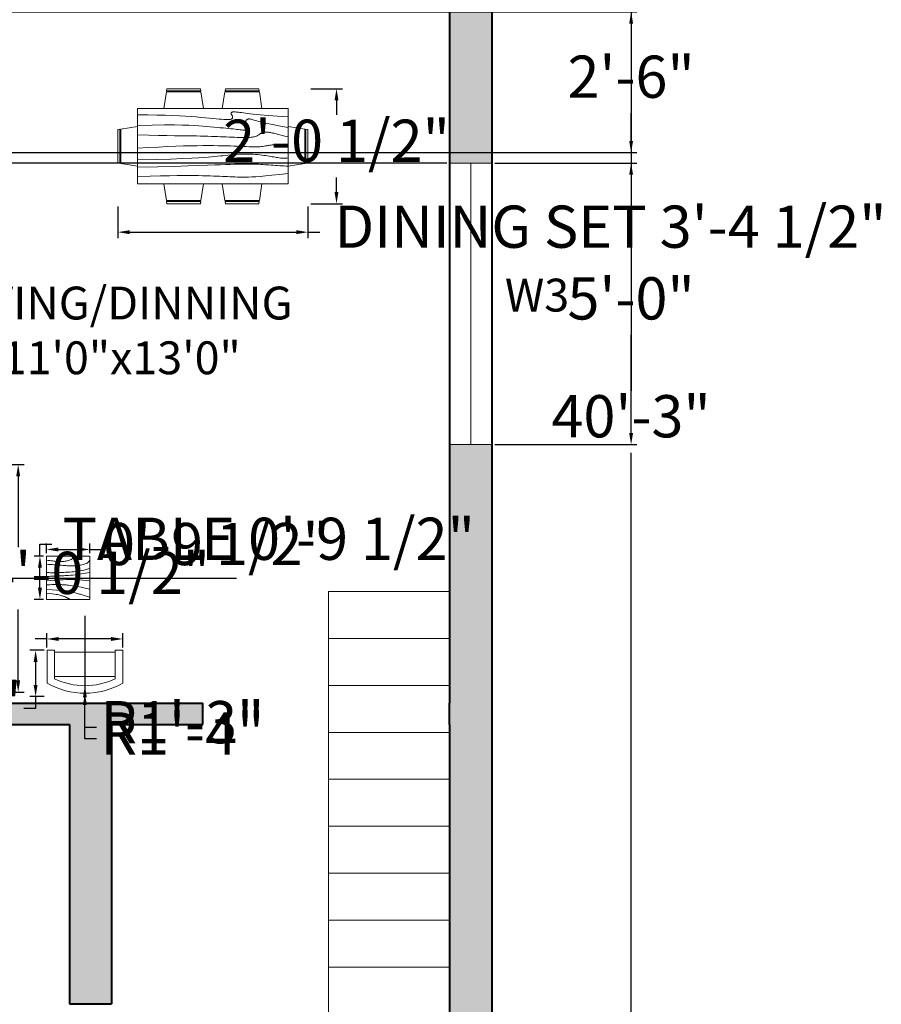
# Model space of a CAD drawing. Units: inches. Extents: x 1883 to 2353, y 1976 to 2541.
# Tile 4 of 5: x 2170 to 2353, y 2136 to 2346. Entities that reach past the tile are written whole.
import ezdxf

# ---------------------------------------------------------------- set-up
doc = ezdxf.new("R2010")
doc.units = ezdxf.units.IN
for name, color, linetype, lineweight in [('A-ANNO-DIMS', 2, 'Continuous', 18), ('A-ANNO-TEXT', 7, 'Continuous', 18), ('A-AREA-IDEN', 7, 'Continuous', 18), ('A-FLOR-STRS', 7, 'Continuous', 18), ('A-FURN', 8, 'Continuous', 18), ('A-GLAZ', 4, 'Continuous', 18), ('A-WALL', 7, 'Continuous', 40)]:
    doc.layers.add(name, color=color, linetype=linetype, lineweight=lineweight)
doc.layers.add('A-WALL-PATT', color=67, linetype='Continuous', lineweight=13, true_color=0x727430)
doc.styles.get("Standard").update_dxf_attribs({"font": 'arial.ttf'})
doc.dimstyles.new('ISO-25', dxfattribs={"dimtxt": 9, "dimasz": 2.5, "dimexe": 1.25, "dimexo": 0.625, "dimgap": 2, "dimtad": 0, "dimtih": 1, "dimtoh": 1, "dimdec": 1, "dimlunit": 4, "dimtxsty": 'Standard', "dimcen": 2.5, "dimadec": 0, "dimazin": 0, "dimtfac": 1, "dimtdec": 1, "dimtmove": 0, "dimatfit": 3, "dimfxl": 1, "dimarcsym": 0})

# ---------------------------------------------------------------- blocks, each defined once
blk = doc.blocks.new('Dining Set - 36 x 72 in.')
for p, q in [((-22.2343, 26.00059), (-23.4847, 17.99762)), ((-22.2304, 26), (-5.7608, 26)), ((-22, 27.5), (-22.1562, 26.50042)), ((-5.8416, 26.5), (-22.1534, 26.5)), ((-22, 27.5), (-6, 27.5)), ((-5.8437, 26.49966), (-6, 27.5)), ((-4.5152, 17.99762), (-5.7655, 25.99926)), ((5.7657, 26.00059), (4.5153, 17.99762)), ((5.7696, 26), (22.2392, 26)), ((6, 27.5), (5.8438, 26.50042)), ((22.1584, 26.5), (5.8466, 26.5)), ((6, 27.5), (22, 27.5)), ((22.1563, 26.49966), (22, 27.5)), ((23.4848, 17.99762), (22.2345, 25.99926)), ((36, 18), (-36, 18)), ((-36, 18), (-36, -18)), ((36, -18), (36, 18)), ((-44.0006, 8.23428), (-35.9976, 9.48474)), ((44.0006, 8.23428), (35.9976, 9.48474)), ((-45.5, 8), (-44.5004, 8.15617)), ((-45.5, 8), (-45.5, -8)), ((-44.5, -8.15843), (-44.5, 8.15338)), ((-44, 8.23041), (-44, -8.23915)), ((44, 8.23041), (44, -8.23915)), ((44.5, -8.15843), (44.5, 8.15338)), ((45.5, 8), (44.5005, 8.15617)), ((45.5, 8), (45.5, -8)), ((-44.4997, -8.15631), (-45.5, -8)), ((-35.9976, -9.48476), (-43.9993, -8.2345)), ((35.9976, -9.48476), (43.9993, -8.2345)), ((44.4997, -8.15631), (45.5, -8)), ((-36, -18), (36, -18)), ((-22.2343, -26.0006), (-23.4847, -17.99762)), ((-4.5152, -17.99762), (-5.7655, -25.99928)), ((5.7657, -26.0006), (4.5153, -17.99762)), ((23.4848, -17.99762), (22.2345, -25.99928)), ((-22.2304, -26), (-5.7608, -26)), ((-22, -27.5), (-22.1562, -26.50044)), ((-5.8416, -26.5), (-22.1534, -26.5)), ((-22, -27.5), (-6, -27.5)), ((-5.8437, -26.49967), (-6, -27.5)), ((5.7696, -26), (22.2392, -26)), ((6, -27.5), (5.8438, -26.50044)), ((22.1584, -26.5), (5.8466, -26.5)), ((6, -27.5), (22, -27.5)), ((22.1563, -26.49967), (22, -27.5))]:
    blk.add_line(p, q)
for points in [[(-36, 15), (-31.1772, 14.97754), (-26.8079, 14.91406), (-22.8538, 14.81543), (-19.276, 14.6875), (-16.0362, 14.53613), (-13.0957, 14.36718), (-10.4159, 14.18652), (-7.9583, 14), (-5.6904, 13.81315), (-3.6035, 13.63021), (-1.6954, 13.45508), (0.0365, 13.29166), (1.5945, 13.14388), (2.9811, 13.01562), (4.1988, 12.9108), (5.25, 12.83333), (6.1393, 12.78613), (6.8802, 12.76823), (7.4883, 12.77767), (7.9792, 12.8125), (8.3685, 12.87077), (8.6719, 12.95052), (8.9049, 13.0498), (9.0833, 13.16666), (9.2205, 13.29899), (9.3216, 13.44401), (9.3895, 13.59879), (9.4271, 13.76041), (9.4373, 13.92594), (9.4232, 14.09245), (9.3875, 14.257), (9.3333, 14.41666), (9.2638, 14.56917), (9.1836, 14.71484), (9.0975, 14.85465), (9.0104, 14.98958), (8.9272, 15.1206), (8.8529, 15.2487), (8.7922, 15.37483), (8.75, 15.5), (8.7305, 15.62467), (8.7344, 15.74739), (8.7617, 15.86621), (8.8125, 15.97916), (8.8867, 16.08431), (8.9844, 16.17968), (9.1055, 16.26334), (9.25, 16.33333), (9.4189, 16.38802), (9.6172, 16.42708), (9.8506, 16.45052), (10.125, 16.45833), (10.4463, 16.45052), (10.8203, 16.42708), (11.2529, 16.38802), (11.75, 16.33333), (12.3184, 16.26318), (12.9694, 16.17838), (13.7151, 16.07991), (14.5677, 15.96875), (15.5395, 15.84586), (16.6426, 15.71224), (17.8893, 15.56884), (19.2917, 15.41666), (20.859, 15.25667), (22.5879, 15.08984), (24.4721, 14.91715), (26.5052, 14.73958), (28.6809, 14.5581), (30.9929, 14.3737), (33.4347, 14.18733), (36, 14)], [(-36, 10), (-28.9766, 10.14274), (-23.1725, 10.20442), (-18.4241, 10.19775), (-14.5677, 10.13541), (-11.4399, 10.03011), (-8.877, 9.89453), (-6.7154, 9.74137), (-4.7917, 9.58333), (-2.9698, 9.43082), (-1.2246, 9.28515), (0.4415, 9.14534), (2.026, 9.01041), (3.5266, 8.87939), (4.9408, 8.7513), (6.266, 8.62516), (7.5, 8.5), (8.6411, 8.37549), (9.6914, 8.2539), (10.6538, 8.13818), (11.5312, 8.03125), (12.3267, 7.93603), (13.043, 7.85547), (13.6831, 7.79248), (14.25, 7.75), (14.7471, 7.7303), (15.1797, 7.73307), (15.5537, 7.75732), (15.875, 7.80208), (16.1494, 7.86637), (16.3828, 7.94922), (16.5811, 8.04964), (16.75, 8.16666), (16.8944, 8.29915), (17.0143, 8.44531), (17.1089, 8.60319), (17.1771, 8.77083), (17.218, 8.94629), (17.2305, 9.1276), (17.2137, 9.31282), (17.1667, 9.5), (17.0895, 9.6875), (16.987, 9.875), (16.8649, 10.0625), (16.7292, 10.25), (16.5856, 10.4375), (16.4401, 10.625), (16.2985, 10.8125), (16.1667, 11), (16.05, 11.18733), (15.9518, 11.3737), (15.8752, 11.5581), (15.8229, 11.73958), (15.798, 11.91715), (15.8034, 12.08984), (15.842, 12.25667), (15.9167, 12.41666), (16.0295, 12.56836), (16.1784, 12.70833), (16.3605, 12.83268), (16.5729, 12.9375), (16.8127, 13.01888), (17.0768, 13.07291), (17.3625, 13.0957), (17.6667, 13.08333), (17.9894, 13.03312), (18.3418, 12.94726), (18.7382, 12.82918), (19.1927, 12.68229), (19.7195, 12.51001), (20.3327, 12.31575), (21.0465, 12.10294), (21.875, 11.875), (22.8357, 11.63354), (23.959, 11.37304), (25.2786, 11.08618), (26.8282, 10.76562), (28.6414, 10.40405), (30.752, 9.99414), (33.1936, 9.52856), (36, 9)], [(-36, 5.5), (-30.7157, 5.3348), (-26.069, 5.20963), (-21.9946, 5.11767), (-18.4271, 5.05208), (-15.3009, 5.00602), (-12.5508, 4.97265), (-10.1112, 4.94515), (-7.9167, 4.91666), (-5.909, 4.88167), (-4.0586, 4.83984), (-2.3429, 4.79215), (-0.7396, 4.73958), (0.7739, 4.6831), (2.22, 4.6237), (3.6213, 4.56233), (5, 4.5), (6.373, 4.43782), (7.7344, 4.3776), (9.0723, 4.32129), (10.375, 4.27083), (11.6309, 4.22819), (12.8281, 4.19531), (13.9551, 4.17415), (15, 4.16666), (15.954, 4.17448), (16.819, 4.19791), (17.6001, 4.23698), (18.3021, 4.29166), (18.9299, 4.36198), (19.4883, 4.44791), (19.9823, 4.54948), (20.4167, 4.66666), (20.7969, 4.79899), (21.1302, 4.94401), (21.4245, 5.09879), (21.6875, 5.26041), (21.9271, 5.42594), (22.1511, 5.59245), (22.3672, 5.757), (22.5834, 5.91666), (22.8065, 6.06868), (23.0404, 6.21093), (23.2879, 6.34147), (23.5521, 6.45833), (23.8358, 6.55957), (24.142, 6.64323), (24.4735, 6.70735), (24.8334, 6.75), (25.2235, 6.76969), (25.642, 6.76692), (26.0858, 6.74267), (26.5521, 6.69791), (27.0379, 6.63362), (27.5404, 6.55078), (28.0565, 6.45036), (28.5834, 6.33333), (29.1242, 6.19987), (29.7071, 6.04687), (30.3661, 5.87044), (31.1354, 5.66666), (32.0493, 5.43164), (33.142, 5.16146), (34.4475, 4.85221), (36, 4.5)], [(-36, -1), (-30.7915, -0.6591), (-26.0195, -0.38216), (-21.6519, -0.16284), (-17.6563, 0.00521), (-14.0005, 0.12833), (-10.6523, 0.21289), (-7.5796, 0.26522), (-4.75, 0.29166), (-2.134, 0.29793), (0.2878, 0.28711), (2.5317, 0.26163), (4.6146, 0.22396), (6.5529, 0.17651), (8.3633, 0.12174), (10.0623, 0.06209), (11.6667, 0), (13.1899, -0.06201), (14.6341, -0.1211), (15.9982, -0.17432), (17.2813, -0.21875), (18.4823, -0.25147), (19.6003, -0.26953), (20.6343, -0.27002), (21.5834, -0.25), (22.4481, -0.20768), (23.2357, -0.14584), (23.9549, -0.06836), (24.6146, 0.02083), (25.2235, 0.11784), (25.7904, 0.21875), (26.3241, 0.31966), (26.8334, 0.41666), (27.3265, 0.50618), (27.8099, 0.58593), (28.2894, 0.65397), (28.7709, 0.70833), (29.2601, 0.74707), (29.763, 0.76823), (30.2855, 0.76985), (30.8334, 0.75), (31.4088, 0.70784), (31.9994, 0.64713), (32.589, 0.57275), (33.1615, 0.48958), (33.7008, 0.4025), (34.1908, 0.3164), (34.6153, 0.23616), (34.9584, 0.16666), (35.2099, 0.11165), (35.3848, 0.07031), (35.504, 0.04069), (35.5886, 0.02083), (35.6594, 0.00879), (35.7377, 0.0026), (35.8442, 0.00032), (36, 0)], [(-36, -6.5), (-27.1843, -6.31267), (-20.084, -6.1263), (-14.469, -5.9419), (-10.1094, -5.76042), (-6.7752, -5.58285), (-4.2363, -5.41016), (-2.2629, -5.24333), (-0.625, -5.08334), (0.8708, -4.93099), (2.2715, -4.78646), (3.5872, -4.64974), (4.8281, -4.52084), (6.0046, -4.39974), (7.127, -4.28646), (8.2053, -4.18099), (9.25, -4.08334), (10.2705, -3.99382), (11.2734, -3.91407), (12.2647, -3.84603), (13.25, -3.79167), (14.2354, -3.75293), (15.2266, -3.73177), (16.2295, -3.73015), (17.25, -3.75), (18.2912, -3.79248), (19.3451, -3.85547), (20.4009, -3.93604), (21.4479, -4.03125), (22.4754, -4.13819), (23.4727, -4.25391), (24.4289, -4.37549), (25.3334, -4.5), (26.1785, -4.62492), (26.9694, -4.74935), (27.7145, -4.87281), (28.4219, -4.99479), (29.1, -5.11483), (29.7572, -5.23242), (30.4016, -5.34709), (31.0417, -5.45834), (31.6837, -5.56437), (32.3262, -5.65821), (32.9658, -5.73153), (33.599, -5.77604), (34.2224, -5.78345), (34.8327, -5.74545), (35.4264, -5.65373), (36, -5.5)], [(-36, -10), (-26.4022, -9.81299), (-18.4675, -9.62891), (-11.9839, -9.45069), (-6.7396, -9.28125), (-2.5226, -9.12354), (0.8789, -8.98047), (3.6769, -8.85498), (6.0833, -8.75), (8.2767, -8.66765), (10.3021, -8.60677), (12.1712, -8.56543), (13.8958, -8.54167), (15.4876, -8.53353), (16.9583, -8.53907), (18.3197, -8.55632), (19.5834, -8.58334), (20.7616, -8.61841), (21.8685, -8.66081), (22.9188, -8.71004), (23.9271, -8.76563), (24.9081, -8.82707), (25.8763, -8.89388), (26.8465, -8.96558), (27.8334, -9.04167), (28.8474, -9.12118), (29.8828, -9.20117), (30.93, -9.27824), (31.9792, -9.34896), (33.0205, -9.40991), (34.0443, -9.45768), (35.0407, -9.48885), (36, -9.5)], [(-36, -14.5), (-30.0881, -14.33513), (-25.0332, -14.21224), (-20.7312, -14.12647), (-17.0781, -14.07292), (-13.97, -14.04671), (-11.3027, -14.04297), (-8.9724, -14.05681), (-6.875, -14.08334), (-4.9224, -14.11833), (-3.0905, -14.16016), (-1.3709, -14.20785), (0.2448, -14.26042), (1.7647, -14.3169), (3.1973, -14.3763), (4.5507, -14.43767), (5.8333, -14.5), (7.0554, -14.5621), (8.235, -14.62175), (9.3922, -14.67652), (10.5469, -14.72396), (11.7192, -14.76164), (12.929, -14.78711), (14.1965, -14.79794), (15.5417, -14.79167), (16.9933, -14.76424), (18.6152, -14.70508), (20.4804, -14.60197), (22.6615, -14.44271), (25.2312, -14.21509), (28.2624, -13.9069), (31.8277, -13.50594), (36, -13)]]:
    blk.add_lwpolyline(points)
blk = doc.blocks.new('Sofa - Roundback Loveseat 5 ft.')
for p, q in [((0, -32.44198), (0, -5.99998)), ((-24, -33.99998), (-24, -11.46958)), ((-23.9998, -13.38178), (23.99986, -13.38178)), ((24.00004, -33.99998), (24.00004, -11.46958)), ((-24, -32.44198), (24.00004, -32.44198))]:
    blk.add_line(p, q)
for points in [[(-24, -33.99998), (-30, -33.99998), (-30, -7.99998)], [(30.00004, -7.99998), (30.00004, -33.99998), (24.00004, -33.99998)]]:
    blk.add_lwpolyline(points)
for centre, radius, start, end in [((0, -60.24998), 60.24998, 60.13715, 119.8628), ((0, -61.38438), 55.38444, 64.32083, 115.6792)]:
    blk.add_arc(centre, radius, start, end)
blk = doc.blocks.new('Table - Square Woodgrain 42 x 42 in.')
blk.add_line((0, -42), (42, -42))
for points in [[(0, -4), (1.704, -4.2172), (3.2358, -4.4188), (4.615, -4.604), (5.8615, -4.7721), (6.9951, -4.9224), (8.0357, -5.0541), (9.0031, -5.1667), (9.9171, -5.2594), (10.7951, -5.3316), (11.6445, -5.3836), (12.4702, -5.4157), (13.277, -5.4283), (14.0698, -5.4217), (14.8535, -5.3964), (15.6331, -5.3526), (16.4133, -5.2908), (17.1986, -5.2103), (17.9913, -5.1062), (18.793, -4.9727), (19.6056, -4.8038), (20.4307, -4.5937), (21.2701, -4.3365), (22.1256, -4.0262), (22.9989, -3.6571), (23.888, -3.2272), (24.7756, -2.7516), (25.6408, -2.2491), (26.4624, -1.7387), (27.2195, -1.2395), (27.891, -0.7703), (28.456, -0.3501), (28.8934, 0.002)], [(0, -42), (0, 0), (42, 0), (42, -42)], [(0, -8), (1.8203, -8.1001), (3.6741, -8.2149), (5.5411, -8.3408), (7.4011, -8.4741), (9.2339, -8.6112), (11.0193, -8.7484), (12.7371, -8.8821), (14.3671, -9.0086), (15.8954, -9.1246), (17.3337, -9.2278), (18.6997, -9.3159), (20.0116, -9.387), (21.2871, -9.4389), (22.5442, -9.4696), (23.8008, -9.477), (25.0749, -9.459), (26.3791, -9.4137), (27.7049, -9.3403), (29.0383, -9.2382), (30.3655, -9.1068), (31.6728, -8.9455), (32.9461, -8.7535), (34.1717, -8.5304), (35.3358, -8.2756), (36.4268, -7.9863), (37.443, -7.6521), (38.3849, -7.2603), (39.253, -6.7986), (40.048, -6.2542), (40.7705, -5.6147), (41.421, -4.8674), (42, -4)], [(42, -12), (39.1784, -12.8621), (36.4519, -13.5654), (33.8246, -14.1294), (31.3004, -14.5731), (28.8832, -14.9161), (26.577, -15.1775), (24.3858, -15.3768), (22.3136, -15.5332), (20.3622, -15.6632), (18.5254, -15.7718), (16.7947, -15.8612), (15.1618, -15.9338), (13.6183, -15.9916), (12.1558, -16.0369), (10.7659, -16.0718), (9.4403, -16.0987), (8.1703, -16.1191), (6.9461, -16.1325), (5.7577, -16.1377), (4.595, -16.1335), (3.4479, -16.1188), (2.3064, -16.0924), (1.1604, -16.0532), (0, -16)], [(42, -16), (37.6529, -16.7365), (33.8802, -17.329), (30.6179, -17.7961), (27.8015, -18.1561), (25.3668, -18.4275), (23.2497, -18.6288), (21.3859, -18.7785), (19.7111, -18.8949), (18.1693, -18.9939), (16.7375, -19.0795), (15.401, -19.1534), (14.1449, -19.217), (12.9544, -19.2717), (11.8148, -19.3191), (10.7113, -19.3606), (9.6291, -19.3976), (8.5534, -19.4323), (7.47, -19.4689), (6.3643, -19.5122), (5.222, -19.5672), (4.0288, -19.6386), (2.7703, -19.7313), (1.4321, -19.8501), (0, -20)], [(0, -24), (3.9243, -23.6805), (7.4766, -23.4138), (10.6891, -23.1954), (13.5943, -23.0205), (16.2247, -22.8847), (18.6125, -22.7832), (20.7903, -22.7116), (22.7903, -22.6651), (24.6563, -22.642), (26.4764, -22.6507), (28.35, -22.7024), (30.3766, -22.8084), (32.6555, -22.98), (35.2861, -23.2283), (38.3678, -23.5645), (42, -24)], [(42, -32), (37.392, -31.017), (33.4585, -30.2231), (30.1291, -29.5949), (27.3334, -29.109), (25.0009, -28.742), (23.0612, -28.4707), (21.4439, -28.2716), (20.0786, -28.1215), (18.8998, -28.0002), (17.8609, -27.9014), (16.9206, -27.8219), (16.0371, -27.7588), (15.1691, -27.709), (14.2748, -27.6693), (13.3128, -27.6368), (12.2415, -27.6083), (11.0295, -27.5824), (9.6867, -27.5643), (8.233, -27.5608), (6.6884, -27.5787), (5.0728, -27.6248), (3.4062, -27.7058), (1.7086, -27.8286), (0, -28)], [(0, -32), (5.4026, -32.5358), (9.9494, -33.019), (13.7424, -33.4553), (16.8834, -33.8505), (19.4743, -34.2106), (21.6171, -34.5413), (23.4136, -34.8486), (24.9657, -35.1382), (26.3614, -35.4156), (27.6332, -35.6841), (28.7995, -35.9467), (29.8788, -36.2064), (30.8897, -36.4661), (31.8507, -36.7288), (32.7802, -36.9973), (33.6968, -37.2747), (34.6175, -37.5635), (35.5531, -37.8651), (36.5128, -38.1805), (37.506, -38.5108), (38.5421, -38.8568), (39.6302, -39.2197), (40.7797, -39.6004), (42, -40)], [(0, -36), (3.0098, -36.2857), (5.5354, -36.5643), (7.6368, -36.8359), (9.374, -37.1009), (10.807, -37.3597), (11.9957, -37.6126), (13.0002, -37.8599), (13.8804, -38.102), (14.6874, -38.3393), (15.4365, -38.5729), (16.1338, -38.8041), (16.7858, -39.0341), (17.3987, -39.264), (17.9787, -39.4952), (18.5322, -39.7288), (19.0655, -39.9662), (19.5832, -40.2081), (20.0842, -40.4544), (20.5657, -40.7046), (21.0249, -40.9581), (21.459, -41.2144), (21.8653, -41.4731), (22.2409, -41.7335), (22.5831, -41.9951)]]:
    blk.add_lwpolyline(points)
blk = doc.blocks.new('*D31')
at = {"layer": 'A-ANNO-DIMS', "color": 0, "lineweight": -2, "transparency": 16777216}
for p, q in [((2190.81, 2306.42), (2190.81, 2299.72)), ((2231.31, 2306.42), (2231.31, 2299.72)), ((2193.31, 2300.97), (2228.81, 2300.97)), ((2231.31, 2300.97), (2233.81, 2300.97))]:
    blk.add_line(p, q, dxfattribs=at)
at = {"layer": 'A-ANNO-DIMS', "color": 0, "transparency": 16777216}
for points in [[(2193.31, 2301.38), (2193.31, 2300.55), (2190.81, 2300.97)], [(2228.81, 2301.38), (2228.81, 2300.55), (2231.31, 2300.97)]]:
    blk.add_solid(points, dxfattribs=at)
at = {"layer": 'Defpoints', "color": 0, "transparency": 16777216}
for p in [(2190.81, 2307.04), (2231.31, 2307.04), (2231.31, 2300.97)]:
    blk.add_point(p, dxfattribs=at)
at = {"layer": 'A-ANNO-DIMS', "color": 0, "transparency": 16777216, "insert": (2295.76, 2300.97), "char_height": 9, "attachment_point": 5}
blk.add_mtext('DINING SET 3\'-4 1/2"', dxfattribs=at)
blk = doc.blocks.new('*D32')
at = {"layer": 'A-ANNO-DIMS', "color": 0, "lineweight": -2, "transparency": 16777216}
for p, q in [((2231.94, 2331.53), (2238.64, 2331.53)), ((2237.39, 2329.03), (2237.39, 2325.94)), ((2237.39, 2309.54), (2237.39, 2312.63)), ((2231.94, 2307.04), (2238.64, 2307.04))]:
    blk.add_line(p, q, dxfattribs=at)
at = {"layer": 'A-ANNO-DIMS', "color": 0, "transparency": 16777216}
for points in [[(2236.97, 2329.03), (2237.81, 2329.03), (2237.39, 2331.53)], [(2236.97, 2309.54), (2237.81, 2309.54), (2237.39, 2307.04)]]:
    blk.add_solid(points, dxfattribs=at)
at = {"layer": 'Defpoints', "color": 0, "transparency": 16777216}
for p in [(2231.31, 2331.53), (2237.39, 2331.53), (2231.31, 2307.04)]:
    blk.add_point(p, dxfattribs=at)
at = {"layer": 'A-ANNO-DIMS', "color": 0, "transparency": 16777216, "insert": (2237.39, 2319.28), "char_height": 9, "attachment_point": 5}
blk.add_mtext('2\'-0 1/2"', dxfattribs=at)
blk = doc.blocks.new('*D33')
at = {"layer": 'A-ANNO-DIMS', "color": 0, "lineweight": -2, "transparency": 16777216}
for p, q in [((2162.94, 2251.43), (2170.84, 2251.43)), ((2169.59, 2248.93), (2169.59, 2233.85)), ((2169.59, 2205.45), (2169.59, 2220.53)), ((2162.94, 2202.95), (2170.84, 2202.95))]:
    blk.add_line(p, q, dxfattribs=at)
at = {"layer": 'A-ANNO-DIMS', "color": 0, "transparency": 16777216}
for points in [[(2169.17, 2248.93), (2170.01, 2248.93), (2169.59, 2251.43)], [(2169.17, 2205.45), (2170.01, 2205.45), (2169.59, 2202.95)]]:
    blk.add_solid(points, dxfattribs=at)
at = {"layer": 'Defpoints', "color": 0, "transparency": 16777216}
for p in [(2162.32, 2251.43), (2169.59, 2251.43), (2162.32, 2202.95)]:
    blk.add_point(p, dxfattribs=at)
at = {"layer": 'A-ANNO-DIMS', "color": 0, "transparency": 16777216, "insert": (2169.59, 2227.19), "char_height": 9, "attachment_point": 5}
blk.add_mtext('SOFA 4\'-0 1/2"', dxfattribs=at)
blk = doc.blocks.new('*D35')
at = {"layer": 'A-ANNO-DIMS', "color": 0, "lineweight": -2, "transparency": 16777216}
for p, q in [((2175.72, 2214.27), (2173.22, 2214.27)), ((2175.72, 2212.47), (2175.72, 2215.52)), ((2189.37, 2214.27), (2178.22, 2214.27)), ((2191.87, 2212.47), (2191.87, 2215.52))]:
    blk.add_line(p, q, dxfattribs=at)
at = {"layer": 'A-ANNO-DIMS', "color": 0, "transparency": 16777216}
for points in [[(2178.22, 2214.69), (2178.22, 2213.85), (2175.72, 2214.27)], [(2189.37, 2214.69), (2189.37, 2213.85), (2191.87, 2214.27)]]:
    blk.add_solid(points, dxfattribs=at)
at = {"layer": 'Defpoints', "color": 0, "transparency": 16777216}
for p in [(2175.72, 2214.27), (2175.72, 2211.85), (2191.87, 2211.85)]:
    blk.add_point(p, dxfattribs=at)
at = {"layer": 'A-ANNO-DIMS', "color": 0, "transparency": 16777216, "insert": (2124.52, 2214.27), "char_height": 9, "attachment_point": 5}
blk.add_mtext('LOVESEAT 1\'-4"', dxfattribs=at)
blk = doc.blocks.new('*D36')
at = {"layer": 'A-ANNO-DIMS', "color": 0, "lineweight": -2, "transparency": 16777216}
for p, q in [((2175.1, 2211.85), (2172.05, 2211.85)), ((2173.3, 2209.35), (2173.3, 2204.48)), ((2175.1, 2201.98), (2172.05, 2201.98)), ((2173.3, 2201.98), (2173.3, 2199.48)), ((2173.3, 2199.48), (2170.8, 2199.48))]:
    blk.add_line(p, q, dxfattribs=at)
at = {"layer": 'A-ANNO-DIMS', "color": 0, "transparency": 16777216}
for points in [[(2172.88, 2209.35), (2173.72, 2209.35), (2173.3, 2211.85)], [(2172.88, 2204.48), (2173.72, 2204.48), (2173.3, 2201.98)]]:
    blk.add_solid(points, dxfattribs=at)
at = {"layer": 'Defpoints', "color": 0, "transparency": 16777216}
for p in [(2175.72, 2211.85), (2173.3, 2201.98), (2175.72, 2201.98)]:
    blk.add_point(p, dxfattribs=at)
at = {"layer": 'A-ANNO-DIMS', "color": 0, "transparency": 16777216, "insert": (2153.34, 2199.48), "char_height": 9, "attachment_point": 5}
blk.add_mtext('0\'-10"', dxfattribs=at)
blk = doc.blocks.new('*D37')
at = {"layer": 'A-ANNO-DIMS', "color": 0, "lineweight": -2, "transparency": 16777216}
for p, q in [((2174.22, 2231.95), (2174.22, 2234.45)), ((2174.22, 2234.45), (2176.72, 2234.45)), ((2174.99, 2231.95), (2172.97, 2231.95)), ((2174.22, 2225.19), (2174.22, 2229.45)), ((2174.99, 2222.69), (2172.97, 2222.69))]:
    blk.add_line(p, q, dxfattribs=at)
at = {"layer": 'A-ANNO-DIMS', "color": 0, "transparency": 16777216}
for points in [[(2173.8, 2229.45), (2174.64, 2229.45), (2174.22, 2231.95)], [(2173.8, 2225.19), (2174.64, 2225.19), (2174.22, 2222.69)]]:
    blk.add_solid(points, dxfattribs=at)
at = {"layer": 'Defpoints', "color": 0, "transparency": 16777216}
for p in [(2174.22, 2231.95), (2175.61, 2231.95), (2175.61, 2222.69)]:
    blk.add_point(p, dxfattribs=at)
at = {"layer": 'A-ANNO-DIMS', "color": 0, "transparency": 16777216, "insert": (2222.94, 2234.45), "char_height": 9, "attachment_point": 5}
blk.add_mtext('TABLE 0\'-9 1/2"', dxfattribs=at)
blk = doc.blocks.new('*D38')
at = {"layer": 'A-ANNO-DIMS', "color": 0, "lineweight": -2, "transparency": 16777216}
for p, q in [((2175.61, 2232.58), (2175.61, 2234.59)), ((2178.11, 2233.34), (2182.37, 2233.34)), ((2184.87, 2232.58), (2184.87, 2234.59)), ((2184.87, 2233.34), (2187.37, 2233.34))]:
    blk.add_line(p, q, dxfattribs=at)
at = {"layer": 'A-ANNO-DIMS', "color": 0, "transparency": 16777216}
for points in [[(2178.11, 2233.76), (2178.11, 2232.93), (2175.61, 2233.34)], [(2182.37, 2233.76), (2182.37, 2232.93), (2184.87, 2233.34)]]:
    blk.add_solid(points, dxfattribs=at)
at = {"layer": 'Defpoints', "color": 0, "transparency": 16777216}
for p in [(2184.87, 2233.34), (2175.61, 2231.95), (2184.87, 2231.95)]:
    blk.add_point(p, dxfattribs=at)
at = {"layer": 'A-ANNO-DIMS', "color": 0, "transparency": 16777216, "insert": (2211.82, 2233.34), "char_height": 9, "attachment_point": 5}
blk.add_mtext('0\'-9 1/2"', dxfattribs=at)
blk = doc.blocks.new('*D43')
at = {"layer": 'A-ANNO-DIMS', "color": 0, "lineweight": -2, "transparency": 16777216}
for p, q in [((2271.12, 2502.07), (2301.39, 2502.07)), ((2300.14, 2499.57), (2300.14, 2267.17)), ((2300.14, 2021.57), (2300.14, 2253.97)), ((2271.12, 2019.07), (2301.39, 2019.07))]:
    blk.add_line(p, q, dxfattribs=at)
at = {"layer": 'A-ANNO-DIMS', "color": 0, "transparency": 16777216}
for points in [[(2299.73, 2499.57), (2300.56, 2499.57), (2300.14, 2502.07)], [(2299.73, 2021.57), (2300.56, 2021.57), (2300.14, 2019.07)]]:
    blk.add_solid(points, dxfattribs=at)
at = {"layer": 'Defpoints', "color": 0, "transparency": 16777216}
for p in [(2270.49, 2502.07), (2300.14, 2502.07), (2270.49, 2019.07)]:
    blk.add_point(p, dxfattribs=at)
at = {"layer": 'A-ANNO-DIMS', "color": 0, "transparency": 16777216, "insert": (2300.14, 2260.57), "char_height": 9, "attachment_point": 5}
blk.add_mtext('40\'-3"', dxfattribs=at)
blk = doc.blocks.new('*D47')
at = {"layer": 'A-ANNO-DIMS', "color": 0, "lineweight": -2, "transparency": 16777216}
for p, q in [((2271.12, 2315.69), (2301.39, 2315.69)), ((2300.14, 2313.19), (2300.14, 2292.28)), ((2300.14, 2258.19), (2300.14, 2279.09)), ((2271.12, 2255.69), (2301.39, 2255.69))]:
    blk.add_line(p, q, dxfattribs=at)
at = {"layer": 'A-ANNO-DIMS', "color": 0, "transparency": 16777216}
for points in [[(2299.73, 2313.19), (2300.56, 2313.19), (2300.14, 2315.69)], [(2299.73, 2258.19), (2300.56, 2258.19), (2300.14, 2255.69)]]:
    blk.add_solid(points, dxfattribs=at)
at = {"layer": 'Defpoints', "color": 0, "transparency": 16777216}
for p in [(2270.49, 2315.69), (2300.14, 2315.69), (2270.49, 2255.69)]:
    blk.add_point(p, dxfattribs=at)
at = {"layer": 'A-ANNO-DIMS', "color": 0, "transparency": 16777216, "insert": (2300.14, 2285.69), "char_height": 9, "attachment_point": 5}
blk.add_mtext('5\'-0"', dxfattribs=at)
blk = doc.blocks.new('*D48')
at = {"layer": 'A-ANNO-DIMS', "color": 0, "lineweight": -2, "transparency": 16777216}
for p, q in [((2260.87, 2356.57), (1979.44, 2356.57)), ((1980.69, 2354.07), (1980.69, 2342.73)), ((1980.69, 2318.19), (1980.69, 2329.53)), ((2260.87, 2315.69), (1979.44, 2315.69))]:
    blk.add_line(p, q, dxfattribs=at)
at = {"layer": 'A-ANNO-DIMS', "color": 0, "transparency": 16777216}
for points in [[(1980.28, 2354.07), (1981.11, 2354.07), (1980.69, 2356.57)], [(1980.28, 2318.19), (1981.11, 2318.19), (1980.69, 2315.69)]]:
    blk.add_solid(points, dxfattribs=at)
at = {"layer": 'Defpoints', "color": 0, "transparency": 16777216}
for p in [(1980.69, 2356.57), (2261.49, 2356.57), (2261.49, 2315.69)]:
    blk.add_point(p, dxfattribs=at)
at = {"layer": 'A-ANNO-DIMS', "color": 0, "transparency": 16777216, "insert": (1980.69, 2336.13), "char_height": 9, "attachment_point": 5}
blk.add_mtext('3\'-5"', dxfattribs=at)
blk = doc.blocks.new('*D54')
at = {"layer": 'A-ANNO-DIMS', "color": 0, "lineweight": -2, "transparency": 16777216}
for p, q in [((2100.12, 2347.93), (2301.39, 2347.93)), ((2300.14, 2345.43), (2300.14, 2339.52)), ((2300.14, 2320.43), (2300.14, 2326.33)), ((2100.12, 2317.93), (2301.39, 2317.93))]:
    blk.add_line(p, q, dxfattribs=at)
at = {"layer": 'A-ANNO-DIMS', "color": 0, "transparency": 16777216}
for points in [[(2299.73, 2345.43), (2300.56, 2345.43), (2300.14, 2347.93)], [(2299.73, 2320.43), (2300.56, 2320.43), (2300.14, 2317.93)]]:
    blk.add_solid(points, dxfattribs=at)
at = {"layer": 'Defpoints', "color": 0, "transparency": 16777216}
for p in [(2099.49, 2347.93), (2300.14, 2347.93), (2099.49, 2317.93)]:
    blk.add_point(p, dxfattribs=at)
at = {"layer": 'A-ANNO-DIMS', "color": 0, "transparency": 16777216, "insert": (2300.14, 2332.93), "char_height": 9, "attachment_point": 5}
blk.add_mtext('2\'-6"', dxfattribs=at)
blk = doc.blocks.new('*D64')
at = {"layer": 'A-ANNO-DIMS', "color": 0, "lineweight": -2, "transparency": 16777216}
for p, q in [((2104.18, 2227.19), (2143.66, 2227.19)), ((2216.11, 2227.19), (2146.16, 2227.19))]:
    blk.add_line(p, q, dxfattribs=at)
at = {"layer": 'A-ANNO-DIMS', "color": 0, "transparency": 16777216}
blk.add_solid([(2143.66, 2227.61), (2143.66, 2226.77), (2146.16, 2227.19)], dxfattribs=at)
at = {"layer": 'Defpoints', "color": 0, "transparency": 16777216}
for p in [(2146.16, 2227.19), (2216.11, 2227.19)]:
    blk.add_point(p, dxfattribs=at)
at = {"layer": 'A-ANNO-DIMS', "color": 0, "transparency": 16777216, "insert": (2082.42, 2227.19), "char_height": 9, "attachment_point": 5}
blk.add_mtext('R5\'-10"', dxfattribs=at)
blk = doc.blocks.new('*D65')
at = {"layer": 'A-ANNO-DIMS', "color": 0, "lineweight": -2, "transparency": 16777216}
for p, q in [((2103.13, 2227.19), (2140.19, 2227.19)), ((2208.64, 2227.19), (2142.69, 2227.19))]:
    blk.add_line(p, q, dxfattribs=at)
at = {"layer": 'A-ANNO-DIMS', "color": 0, "transparency": 16777216}
blk.add_solid([(2140.19, 2227.61), (2140.19, 2226.77), (2142.69, 2227.19)], dxfattribs=at)
at = {"layer": 'Defpoints', "color": 0, "transparency": 16777216}
for p in [(2142.69, 2227.19), (2208.64, 2227.19)]:
    blk.add_point(p, dxfattribs=at)
at = {"layer": 'A-ANNO-DIMS', "color": 0, "transparency": 16777216, "insert": (2084.86, 2227.19), "char_height": 9, "attachment_point": 5}
blk.add_mtext('R5\'-6"', dxfattribs=at)
blk = doc.blocks.new('*D66')
at = {"layer": 'A-ANNO-DIMS', "color": 0, "lineweight": -2, "transparency": 16777216}
for p, q in [((2183.8, 2218.91), (2183.8, 2202.7)), ((2183.8, 2192.97), (2183.8, 2200.2)), ((2186.3, 2192.97), (2183.8, 2192.97))]:
    blk.add_line(p, q, dxfattribs=at)
at = {"layer": 'A-ANNO-DIMS', "color": 0, "transparency": 16777216}
blk.add_solid([(2184.21, 2200.2), (2183.38, 2200.2), (2183.8, 2202.7)], dxfattribs=at)
at = {"layer": 'Defpoints', "color": 0, "transparency": 16777216}
for p in [(2183.8, 2218.91), (2183.8, 2202.7)]:
    blk.add_point(p, dxfattribs=at)
at = {"layer": 'A-ANNO-DIMS', "color": 0, "transparency": 16777216, "insert": (2204.57, 2192.97), "char_height": 9, "attachment_point": 5}
blk.add_mtext('R1\'-4"', dxfattribs=at)
blk = doc.blocks.new('*D67')
at = {"layer": 'A-ANNO-DIMS', "color": 0, "lineweight": -2, "transparency": 16777216}
for p, q in [((2183.8, 2219.22), (2183.8, 2204.31)), ((2183.8, 2195.37), (2183.8, 2201.81)), ((2186.3, 2195.37), (2183.8, 2195.37))]:
    blk.add_line(p, q, dxfattribs=at)
at = {"layer": 'A-ANNO-DIMS', "color": 0, "transparency": 16777216}
blk.add_solid([(2184.21, 2201.81), (2183.38, 2201.81), (2183.8, 2204.31)], dxfattribs=at)
at = {"layer": 'Defpoints', "color": 0, "transparency": 16777216}
for p in [(2183.8, 2219.22), (2183.8, 2204.31)]:
    blk.add_point(p, dxfattribs=at)
at = {"layer": 'A-ANNO-DIMS', "color": 0, "transparency": 16777216, "insert": (2204.57, 2195.37), "char_height": 9, "attachment_point": 5}
blk.add_mtext('R1\'-3"', dxfattribs=at)

msp = doc.modelspace()

# ---------------------------------------------------------------- hatches: boundary and pattern name
at = {"layer": 'A-WALL-PATT'}
h = msp.add_hatch(color=256, dxfattribs=at)
h.dxf.hatch_style = 1
h.paths.add_polyline_path([(2057.49, 2502.07), (2006.49, 2502.07), (2006.49, 2344.57), (2015.49, 2344.57), (2015.49, 2356.57), (2099.49, 2356.57), (2099.49, 2347.93), (2103.99, 2347.93), (2103.99, 2356.57), (2108.06, 2356.57, -0.029386), (2108.06, 2361.07), (2015.49, 2361.07), (2015.49, 2493.07), (2057.49, 2493.07)])
h.paths.add_polyline_path([(2182.74, 2502.07), (2105.49, 2502.07), (2105.49, 2493.07), (2147.49, 2493.07), (2147.49, 2361.07), (2144.06, 2361.07), (2144.06, 2356.57), (2151.99, 2356.57), (2155, 2356.57), (2155, 2361.07), (2151.99, 2361.07), (2151.99, 2493.07), (2182.74, 2493.07)])
h.paths.add_polyline_path([(2270.49, 2502.07), (2230.74, 2502.07), (2230.74, 2493.07), (2261.49, 2493.07), (2261.49, 2361.07), (2191, 2361.07, -0.029386), (2191, 2356.57), (2261.49, 2356.57), (2261.49, 2315.69), (2270.49, 2315.69)])
h.paths.add_polyline_path([(2051.49, 2131.57), (2015.49, 2131.57), (2015.49, 2251.57), (2103.99, 2251.57), (2104.81, 2251.57, -0.028441), (2104.81, 2256.07), (2103.99, 2256.07), (2103.99, 2260.88), (2099.49, 2260.88), (2099.49, 2256.07), (2015.49, 2256.07), (2015.49, 2268.07), (2006.49, 2268.07), (2006.49, 2122.57), (2015.49, 2122.57), (2051.49, 2122.57)])
h.paths.add_polyline_path([(2103.99, 2308.57), (2103.99, 2317.93, -0.034841), (2099.49, 2317.93), (2099.49, 2308.57), (2015.49, 2308.57), (2015.49, 2320.57), (2006.49, 2320.57), (2006.49, 2292.07), (2015.49, 2292.07), (2015.49, 2304.07), (2099.49, 2304.07), (2099.49, 2290.88, -0.034841), (2103.99, 2290.88), (2103.99, 2304.07)])
h = msp.add_hatch(color=256, dxfattribs=at)
h.dxf.hatch_style = 1
h.paths.add_polyline_path([(2189.49, 2090.74), (2180.49, 2090.74), (2180.49, 2071.57, -0.034524), (2180.49, 2067.07), (2189.49, 2067.07), (2261.49, 2067.07), (2270.49, 2067.07), (2270.49, 2094.07), (2270.49, 2255.69), (2261.49, 2255.69), (2261.49, 2200.57), (2261.49, 2196.07), (2261.49, 2094.07), (2261.49, 2076.07), (2189.49, 2076.07)])
h.paths.add_polyline_path([(2189.49, 2196.07), (2208.94, 2196.07), (2208.94, 2200.57), (2151.99, 2200.57), (2139.99, 2200.57), (2139.99, 2251.57), (2139.99, 2256.07), (2135.49, 2256.07), (2134.13, 2256.07), (2134.13, 2251.57), (2135.49, 2251.57), (2135.49, 2131.57), (2099.49, 2131.57), (2099.49, 2122.57), (2103.99, 2122.57), (2135.49, 2122.57), (2139.99, 2122.57), (2139.99, 2196.07), (2151.99, 2196.07), (2180.49, 2196.07), (2180.49, 2136.51), (2189.49, 2136.51)])

# ---------------------------------------------------------------- linework, layer by layer
at = {"layer": 'A-FLOR-STRS'}
for p, q in [((2235.72, 2224.36), (2261.49, 2224.36)), ((2235.72, 2221.83), (2235.72, 2224.36)), ((2235.72, 2221.83), (2235.72, 2104.36)), ((2235.72, 2214.36), (2261.49, 2214.36)), ((2235.72, 2204.36), (2261.49, 2204.36)), ((2235.72, 2194.36), (2261.49, 2194.36)), ((2235.72, 2184.36), (2261.49, 2184.36)), ((2235.72, 2174.36), (2261.49, 2174.36)), ((2235.72, 2164.36), (2261.49, 2164.36)), ((2235.72, 2154.36), (2261.49, 2154.36)), ((2235.72, 2144.36), (2261.49, 2144.36))]:
    msp.add_line(p, q, dxfattribs=at)
at = {"layer": 'A-GLAZ'}
for p, q in [((2261.49, 2315.69), (2270.49, 2315.69)), ((2265.99, 2315.69), (2265.99, 2255.69)), ((2261.49, 2255.69), (2270.49, 2255.69))]:
    msp.add_line(p, q, dxfattribs=at)
at = {"layer": 'A-WALL'}
for p, q in [((2270.49, 2502.07), (2270.49, 2094.07)), ((2261.49, 2356.57), (2261.49, 2200.57)), ((2151.99, 2200.57), (2208.94, 2200.57)), ((2208.94, 2196.07), (2208.94, 2200.57)), ((2261.49, 2196.07), (2261.49, 2200.57)), ((2151.99, 2196.07), (2180.49, 2196.07)), ((2180.49, 2196.07), (2180.49, 2136.51)), ((2189.49, 2196.07), (2189.49, 2136.51)), ((2189.49, 2196.07), (2208.94, 2196.07)), ((2261.49, 2196.07), (2261.49, 2094.07)), ((2180.49, 2136.51), (2189.49, 2136.51))]:
    msp.add_line(p, q, dxfattribs=at)

# ---------------------------------------------------------------- block references
at = {"layer": 'A-FURN'}
for name, p, xscale, yscale, zscale in [('Dining Set - 36 x 72 in.', (2211.06, 2319.28), 0.4451605360909625, 0.4451605360909625, 0.4451605360909625), ('Table - Square Woodgrain 42 x 42 in.', (2175.61, 2231.95), 0.2204614999433201, 0.2204614999433201, 0.2204614999433201)]:
    msp.add_blockref(name, p, dxfattribs=dict(at, xscale=xscale, yscale=yscale, zscale=zscale))
at = {"layer": 'A-FURN', "xscale": 0.269144385213627, "yscale": 0.269144385213627, "zscale": 0.269144385213627, "rotation": 180}
msp.add_blockref('Sofa - Roundback Loveseat 5 ft.', (2183.8, 2202.7), dxfattribs=at)

# ---------------------------------------------------------------- texts
at = {"layer": 'A-ANNO-TEXT', "insert": (2273.96, 2291.05), "char_height": 7, "attachment_point": 1}
msp.add_mtext_dynamic_manual_height_columns('\\pxqc;{\\fArial|b1|i0|c0|p34;W3}', width=12.2802, gutter_width=12.5, heights=[0], dxfattribs=at)
at = {"layer": 'A-AREA-IDEN', "insert": (2151.7, 2289.36), "char_height": 7, "attachment_point": 1}
msp.add_mtext_dynamic_manual_height_columns('\\pxqc;{\\fArial|b1|i0|c0|p34;LIVING/DINNING\\P11\'0"x13\'0"}', width=79.6787, gutter_width=12.5, heights=[0], dxfattribs=at)

# ---------------------------------------------------------------- dimensions: what is measured, and where the dimension line sits
at = {"layer": 'A-ANNO-DIMS'}
for base, p1, p2, angle, picture, middle in [((2300.14, 2502.07), (2270.49, 2019.07), (2270.49, 2502.07), 90, '*D43', (2300.14, 2260.57)), ((1980.69, 2356.57), (2261.49, 2315.69), (2261.49, 2356.57), 90, '*D48', (1980.69, 2336.13)), ((2300.14, 2347.93), (2099.49, 2317.93), (2099.49, 2347.93), 90, '*D54', (2300.14, 2332.93)), ((2237.39, 2331.53), (2231.31, 2307.04), (2231.31, 2331.53), 90, '*D32', (2237.39, 2319.28)), ((2300.14, 2315.69), (2270.49, 2255.69), (2270.49, 2315.69), 90, '*D47', (2300.14, 2285.69)), ((2173.3, 2201.98), (2175.72, 2211.85), (2175.72, 2201.98), 270, '*D36', (2153.34, 2199.48))]:
    dim = msp.add_linear_dim(base=base, p1=p1, p2=p2, angle=angle, dimstyle='ISO-25', override={"dimdec": 1, "dimlfac": 1, "dimrnd": 0, "dimzin": 1, "dimdsep": 46, "dimlunit": 4, "dimfrac": 2}, dxfattribs=at)
    dim.commit()
    dim.dimension.update_dxf_attribs({"geometry": picture, "text_midpoint": middle})
dim = msp.add_linear_dim(base=(2231.31, 2300.97), p1=(2190.81, 2307.04), p2=(2231.31, 2307.04), text='DINING SET <>', dimstyle='ISO-25', override={"dimdec": 1, "dimlfac": 1, "dimrnd": 0, "dimzin": 1, "dimdsep": 46, "dimlunit": 4, "dimfrac": 2}, dxfattribs=at)
dim.commit()
dim.dimension.update_dxf_attribs({"geometry": '*D31', "text_midpoint": (2295.76, 2300.97)})
for base, p1, p2, angle, text, picture, middle in [((2174.22, 2231.95), (2175.61, 2222.69), (2175.61, 2231.95), 90, 'TABLE <>', '*D37', (2222.94, 2234.45)), ((2169.59, 2251.43), (2162.32, 2202.95), (2162.32, 2251.43), 90, 'SOFA <>', '*D33', (2169.59, 2227.19)), ((2175.7232, 2214.2703), (2191.8719, 2211.848), (2175.7232, 2211.848), 180, 'LOVESEAT <>', '*D35', (2124.5227, 2214.2703))]:
    dim = msp.add_linear_dim(base=base, p1=p1, p2=p2, angle=angle, text=text, dimstyle='ISO-25', override={"dimdec": 1, "dimlfac": 1, "dimrnd": 0, "dimzin": 1, "dimdsep": 46, "dimlunit": 4, "dimfrac": 2}, dxfattribs=at)
    dim.commit()
    dim.dimension.update_dxf_attribs({"geometry": picture, "text_midpoint": middle})
dim = msp.add_linear_dim(base=(2184.87, 2233.34), p1=(2175.61, 2231.95), p2=(2184.87, 2231.95), dimstyle='ISO-25', override={"dimdec": 1, "dimlfac": 1, "dimrnd": 0, "dimzin": 1, "dimdsep": 46, "dimlunit": 4, "dimfrac": 2}, dxfattribs=at)
dim.commit()
dim.dimension.update_dxf_attribs({"geometry": '*D38', "text_midpoint": (2211.82, 2233.34)})
for center, mpoint, picture, middle in [((2216.1109, 2227.1903), (2146.1566, 2227.19), '*D64', (2104.184, 2227.1898)), ((2208.6381, 2227.1903), (2142.6934, 2227.19), '*D65', (2103.1266, 2227.1898)), ((2183.8, 2219.22), (2183.8, 2204.31), '*D67', (2204.57, 2195.37)), ((2183.8, 2218.91), (2183.8, 2202.7), '*D66', (2204.57, 2192.97))]:
    dim = msp.add_radius_dim(center=center, mpoint=mpoint, dimstyle='ISO-25', override={"dimdec": 1, "dimlfac": 1, "dimrnd": 0, "dimzin": 1, "dimdsep": 46, "dimlunit": 4, "dimfrac": 2}, dxfattribs=at)
    dim.commit()
    dim.dimension.update_dxf_attribs({"geometry": picture, "text_midpoint": middle, "dimtype": 164})

doc.saveas('drawing.dxf')
